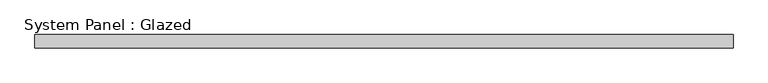
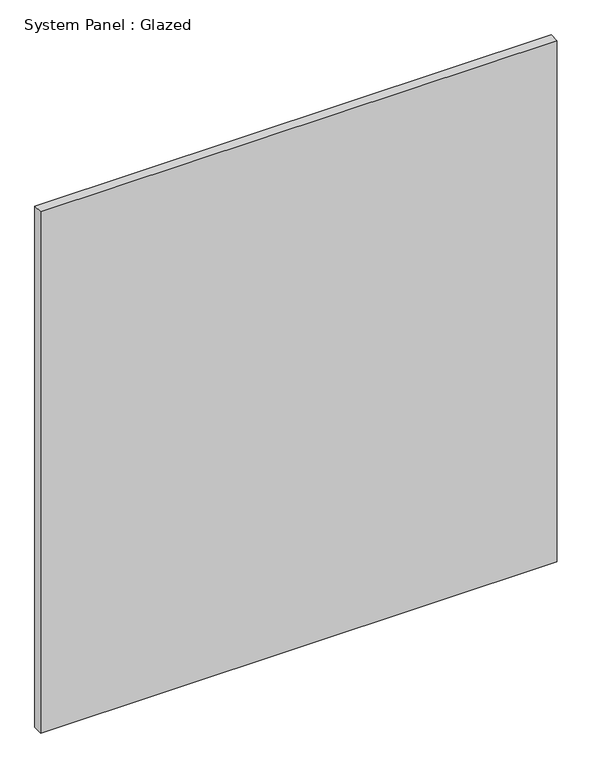
"""IFC4 building model written with IfcOpenShell, lengths in millimetres: plate geometry, System Panel : Glazed."""

from ifc_helpers import new_model, si_unit, origin, origin_with_axes, place, context, project, spatial, polyline, outline, extrude, source, transform, mapped, element, save


def system_panel_glazed_2854df63(model_context):
    return source(origin(), model_context, "Body", "SweptSolid", [
        extrude(outline(polyline([(669.925, 19.05), (-669.925, 19.05), (-669.925, 44.45), (669.925, 44.45), (669.925, 19.05)])), origin_with_axes(), (0.0, 0.0, 1.0), 1428.75),
    ])


if __name__ == "__main__":
    model = new_model("IFC4")
    model_context = context("Model", 3, world=origin())
    ifc_project = project(units=[si_unit("LENGTHUNIT", "METRE", prefix="MILLI")], contexts=[model_context])
    site = spatial("IfcSite", under=ifc_project)
    building = spatial("IfcBuilding", under=site)
    placement = place(None, origin())
    system_panel_glazed_shape = system_panel_glazed_2854df63(model_context)
    element("IfcPlate", 1, ObjectType="System Panel : Glazed", at=placement, inside=building, context=model_context, shape_type="MappedRepresentation", body=[
        mapped(system_panel_glazed_shape, transform((0.0, 0.0, 0.0), x_axis=(1.0, 0.0, 0.0), y_axis=(0.0, 1.0, 0.0), z_axis=(0.0, 0.0, 1.0))),
    ])
    save(model, "model.ifc")

# Revit data of these elements
# Type "System Panel : Glazed"
#   Construction Type Id = "GSP4R"
#   Analytic Construction = "1/8 in Pilkington single glazing"
#   Visual Light Transmittance = 0.9
#   Solar Heat Gain Coefficient = 0.86
#   Heat Transfer Coefficient (U) = 1.18115 BTU/(h·ft²·°F)
#   Define Thermal Properties by = 1
# Element 1 (IfcPlate, "System Panel : Glazed")
#   Materials on its faces: "Glass"
# Materials
#   "Glass": class "Glass", colour RGB 0 128 192, transparency 0.75, Description = "Soda Lime Glass", Cost = 0
